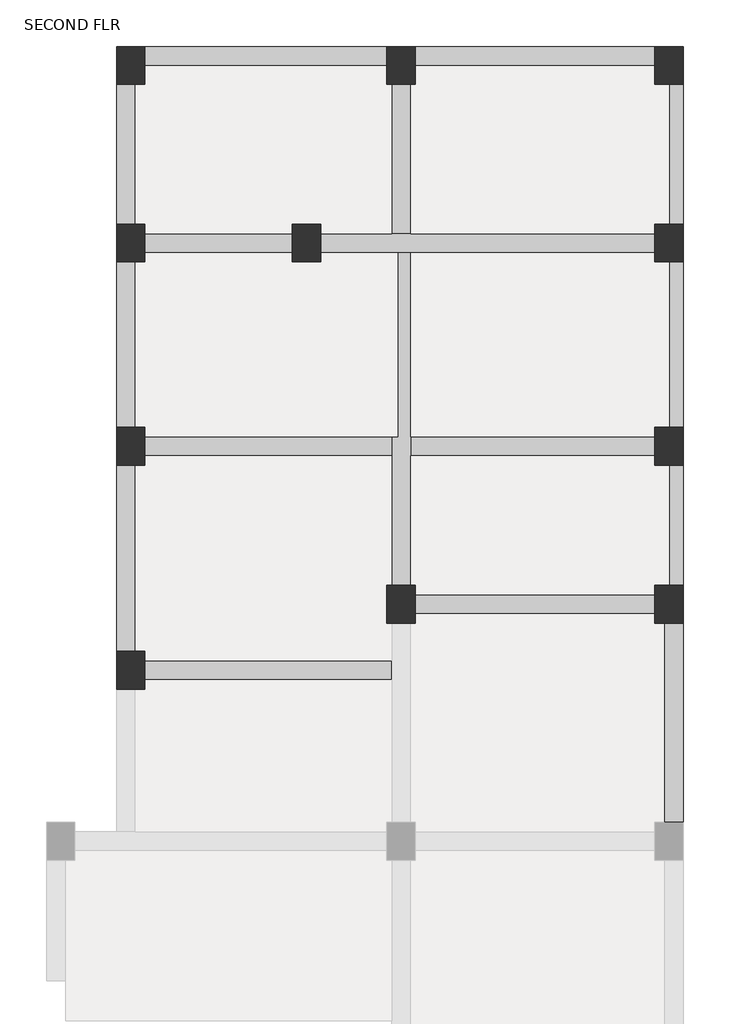
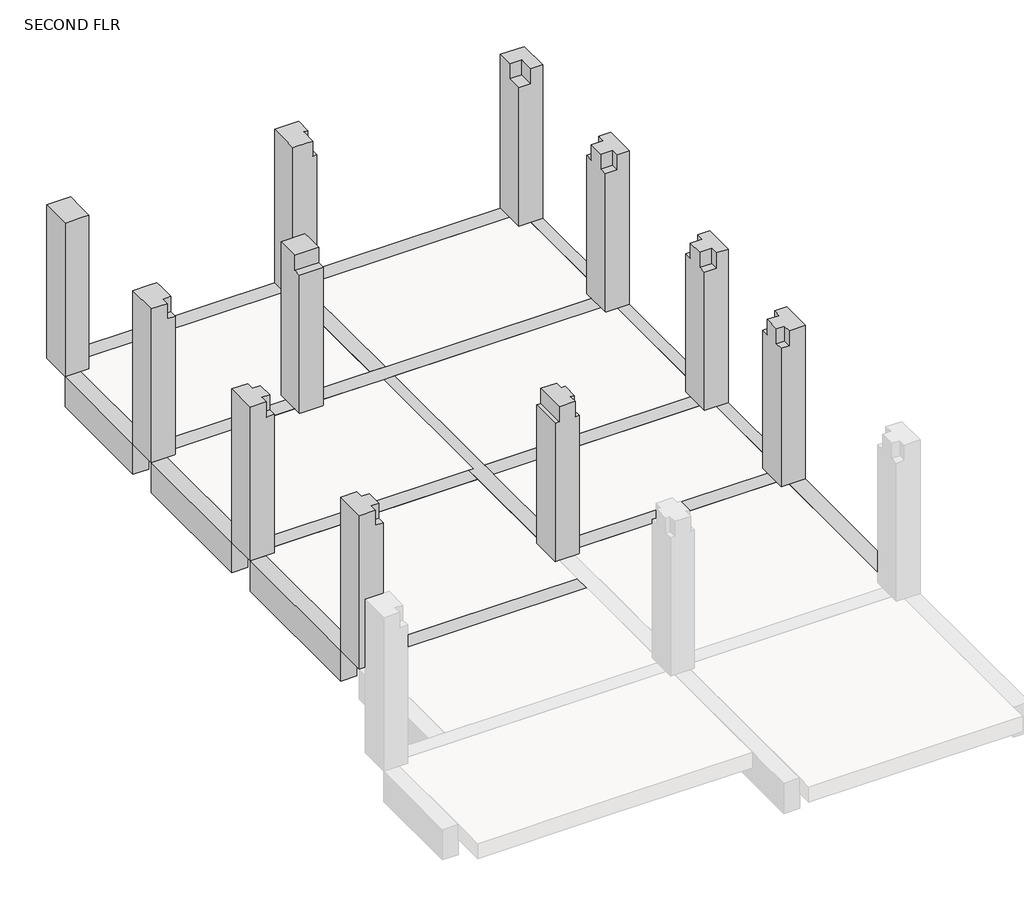
# One storey, part 2 of 2: 17 beams, 11 columns.
"""IFC4 building model written with IfcOpenShell, lengths in millimetres."""

from ifc_helpers import new_model, si_unit, frame, origin, place, context, project, spatial, polyline, outline, extrude, faceted_brep, element, save

model = new_model("IFC4")

# Units and contexts
model_context = context("Model", 3, world=origin())
ifc_project = project(units=[si_unit("LENGTHUNIT", "METRE", prefix="MILLI")], contexts=[model_context])

# Site, building, storey
site = spatial("IfcSite", under=ifc_project)
building = spatial("IfcBuilding", under=site)
storey = spatial("IfcBuildingStorey", under=building, Name="SECOND FLR", Elevation=6048.0)

# Beams
placement = place(None, origin())
element("IfcBeam", 1, ObjectType="M_Concrete-Rectangular Beam : 300 x 600mm", at=placement, inside=storey, context=model_context, shape_type="Brep", body=[
    faceted_brep([(-2096.635935, 10150.0657956, 6048.0), (-2096.635935, 10450.0657956, 6048.0), (-5925.9642664, 10450.0657956, 6048.0), (-5925.9642664, 10150.0657956, 6048.0), (-2096.635935, 10150.0657956, 5448.0), (-2096.635935, 10150.0657956, 5748.0), (-5925.9642664, 10150.0657956, 5748.0), (-5925.9642664, 10150.0657956, 5448.0), (-2096.635935, 10450.0657956, 5448.0), (-5925.9642664, 10450.0657956, 5448.0)], [[[0, 1, 2, 3]], [[4, 5, 0, 3, 6, 7]], [[8, 4, 7, 9]], [[1, 8, 9, 2]], [[2, 9, 7, 6, 3]], [[1, 0, 5, 4, 8]]]),
])
element("IfcBeam", 2, ObjectType="M_Concrete-Rectangular Beam : 300 x 600mm", at=placement, inside=storey, context=model_context, shape_type="SweptSolid", body=[
    extrude(outline(polyline([(2143.5134108, 10450.0657956), (2143.5134108, 10150.0657956), (-1646.635935, 10150.0657956), (-1646.635935, 10450.0657956), (2143.5134108, 10450.0657956)])), frame((0.0, 0.0, 5448.0), z_axis=(0.0, 0.0, 1.0), x_axis=(1.0, 0.0, 0.0)), (0.0, 0.0, 1.0), 600.0),
])
element("IfcBeam", 3, ObjectType="M_Concrete-Rectangular Beam : 300 x 600mm", at=placement, inside=storey, context=model_context, shape_type="Brep", body=[
    faceted_brep([(-6375.9642664, 7641.506653, 6048.0), (-6075.9642664, 7641.506653, 6048.0), (-6075.9642664, 9850.0657956, 6048.0), (-6375.9642664, 9850.0657956, 6048.0), (-6375.9642664, 7641.506653, 5448.0), (-6375.9642664, 9850.0657956, 5448.0), (-6075.9642664, 7641.506653, 5448.0), (-6075.9642664, 9850.0657956, 5448.0), (-6075.9642664, 7641.506653, 5748.0), (-6075.9642664, 9850.0657956, 5748.0)], [[[0, 1, 2, 3]], [[4, 0, 3, 5]], [[6, 4, 5, 7]], [[1, 8, 6, 7, 9, 2]], [[2, 9, 7, 5, 3]], [[1, 0, 4, 6, 8]]]),
])
element("IfcBeam", 4, ObjectType="M_Concrete-Rectangular Beam : 300 x 600mm", at=placement, inside=storey, context=model_context, shape_type="SweptSolid", body=[
    extrude(outline(polyline([(-6075.9642664, 4424.5351605), (-6375.9642664, 4424.5351605), (-6375.9642664, 7041.506653), (-6075.9642664, 7041.506653), (-6075.9642664, 4424.5351605)])), frame((0.0, 0.0, 5448.0), z_axis=(0.0, 0.0, 1.0), x_axis=(1.0, 0.0, 0.0)), (0.0, 0.0, 1.0), 600.0),
])
element("IfcBeam", 5, ObjectType="M_Concrete-Rectangular Beam : 300 x 600mm", at=placement, inside=storey, context=model_context, shape_type="SweptSolid", body=[
    extrude(outline(polyline([(-6075.9642664, 881.5941646), (-6375.9642664, 881.5941646), (-6375.9642664, 3824.5351605), (-6075.9642664, 3824.5351605), (-6075.9642664, 881.5941646)])), frame((0.0, 0.0, 5448.0), z_axis=(0.0, 0.0, 1.0), x_axis=(1.0, 0.0, 0.0)), (0.0, 0.0, 1.0), 600.0),
])
element("IfcBeam", 6, ObjectType="M_Concrete-Rectangular Beam : 300 x 600mm", at=placement, inside=storey, context=model_context, shape_type="SweptSolid", body=[
    extrude(outline(polyline([(2293.5134108, 1328.1057379), (2593.5134108, 1328.1057379), (2593.5134108, -1823.3693625), (2293.5134108, -1823.3693625), (2293.5134108, 1328.1057379)])), frame((0.0, 0.0, 5448.0), z_axis=(0.0, 0.0, 1.0), x_axis=(1.0, 0.0, 0.0)), (0.0, 0.0, 1.0), 600.0),
])
element("IfcBeam", 7, ObjectType="M_Concrete-Rectangular Beam : 300 x 600mm", at=placement, inside=storey, context=model_context, shape_type="SweptSolid", body=[
    extrude(outline(polyline([(5448.0, 2293.5134108), (5448.0, 2593.5134108), (6048.0, 2593.5134108), (6048.0, 2368.5134108), (5748.0, 2368.5134108), (5748.0, 2293.5134108), (5448.0, 2293.5134108)])), frame((0.0, 1928.1057379, 0.0), z_axis=(0.0, 1.0, 0.0), x_axis=(0.0, 0.0, 1.0)), (0.0, 0.0, 1.0), 1896.4294226),
])
element("IfcBeam", 8, ObjectType="M_Concrete-Rectangular Beam : 300 x 600mm", at=placement, inside=storey, context=model_context, shape_type="SweptSolid", body=[
    extrude(outline(polyline([(5448.0, 2293.5134108), (5448.0, 2593.5134108), (6048.0, 2593.5134108), (6048.0, 2368.5134108), (5748.0, 2368.5134108), (5748.0, 2293.5134108), (5448.0, 2293.5134108)])), frame((0.0, 4424.5351605, 0.0), z_axis=(0.0, 1.0, 0.0), x_axis=(0.0, 0.0, 1.0)), (0.0, 0.0, 1.0), 2616.9714925),
])
element("IfcBeam", 9, ObjectType="M_Concrete-Rectangular Beam : 300 x 600mm", at=placement, inside=storey, context=model_context, shape_type="SweptSolid", body=[
    extrude(outline(polyline([(5448.0, 2293.5134108), (5448.0, 2593.5134108), (6048.0, 2593.5134108), (6048.0, 2368.5134108), (5748.0, 2368.5134108), (5748.0, 2293.5134108), (5448.0, 2293.5134108)])), frame((0.0, 7641.506653, 0.0), z_axis=(0.0, 1.0, 0.0), x_axis=(0.0, 0.0, 1.0)), (0.0, 0.0, 1.0), 2208.5591426),
])
element("IfcBeam", 10, ObjectType="M_Concrete-Rectangular Beam : 300 x 600mm", at=placement, inside=storey, context=model_context, shape_type="Brep", body=[
    faceted_brep([(-3596.635935, 7191.506653, 6048.0), (-3596.635935, 7491.506653, 6048.0), (-5925.9642664, 7491.506653, 6048.0), (-5925.9642664, 7191.506653, 6048.0), (-3596.635935, 7191.506653, 5448.0), (-5925.9642664, 7191.506653, 5448.0), (-3596.635935, 7491.506653, 5448.0), (-5925.9642664, 7491.506653, 5448.0), (-3596.635935, 7491.506653, 5748.0), (-5925.9642664, 7491.506653, 5748.0)], [[[0, 1, 2, 3]], [[4, 0, 3, 5]], [[6, 4, 5, 7]], [[1, 8, 6, 7, 9, 2]], [[2, 9, 7, 5, 3]], [[1, 0, 4, 6, 8]]]),
])
element("IfcBeam", 11, ObjectType="M_Concrete-Rectangular Beam : 300 x 600mm", at=placement, inside=storey, context=model_context, shape_type="Brep", body=[
    faceted_brep([(-3146.635935, 7491.506653, 6048.0), (-3146.635935, 7191.506653, 6048.0), (-1928.7254278, 7191.506653, 6048.0), (-1721.635935, 7191.506653, 6048.0), (2143.5134108, 7191.506653, 6048.0), (2143.5134108, 7491.506653, 6048.0), (-1721.635935, 7491.506653, 6048.0), (-2021.635935, 7491.506653, 6048.0), (-3146.635935, 7491.506653, 5448.0), (-3146.635935, 7491.506653, 5748.0), (2143.5134108, 7491.506653, 5448.0), (-1721.635935, 7491.506653, 5448.0), (-2021.635935, 7491.506653, 5448.0), (-3146.635935, 7191.506653, 5448.0), (2143.5134108, 7191.506653, 5448.0), (-1721.635935, 7191.506653, 5448.0), (-2021.635935, 7191.506653, 5448.0)], [[[0, 1, 2, 3, 4, 5, 6, 7]], [[8, 9, 0, 7, 6, 5, 10, 11, 12]], [[13, 8, 12, 11, 10, 14, 15, 16]], [[1, 13, 16, 15, 14, 4, 3, 2]], [[1, 0, 9, 8, 13]], [[4, 14, 10, 5]]]),
])
element("IfcBeam", 12, ObjectType="M_Concrete-Rectangular Beam : 300 x 600mm", at=placement, inside=storey, context=model_context, shape_type="SweptSolid", body=[
    extrude(outline(polyline([(-1646.635935, 1478.1057379), (-1646.635935, 1778.1057379), (2143.5134108, 1778.1057379), (2143.5134108, 1478.1057379), (-1646.635935, 1478.1057379)])), frame((0.0, 0.0, 5448.0), z_axis=(0.0, 0.0, 1.0), x_axis=(1.0, 0.0, 0.0)), (0.0, 0.0, 1.0), 600.0),
])
element("IfcBeam", 13, ObjectType="M_Concrete-Rectangular Beam : 300 x 600mm", at=placement, inside=storey, context=model_context, shape_type="Brep", body=[
    faceted_brep([(-1721.635935, 9850.0657956, 6048.0), (-2021.635935, 9850.0657956, 6048.0), (-2021.635935, 7491.506653, 6048.0), (-1721.635935, 7491.506653, 6048.0), (-2021.635935, 9850.0657956, 5748.0), (-2021.635935, 9850.0657956, 5448.0), (-2021.635935, 7491.506653, 5448.0), (-2021.635935, 7491.506653, 5748.0), (-1721.635935, 9850.0657956, 5448.0), (-1721.635935, 7491.506653, 5448.0), (-1721.635935, 7491.506653, 5748.0)], [[[0, 1, 2, 3]], [[1, 4, 5, 6, 7, 2]], [[5, 8, 9, 6]], [[8, 0, 3, 10, 9]], [[0, 8, 5, 4, 1]], [[3, 2, 7, 6, 9, 10]]]),
])
element("IfcBeam", 14, ObjectType="M_Concrete-Rectangular Beam : 300 x 600mm", at=placement, inside=storey, context=model_context, shape_type="Brep", body=[
    faceted_brep([(-2021.635935, 1928.1057379, 6048.0), (-1721.635935, 1928.1057379, 6048.0), (-1721.635935, 3974.5351605, 6048.0), (-1721.635935, 4274.5351605, 6048.0), (-1721.635935, 7191.506653, 6048.0), (-1928.7254278, 7191.506653, 6048.0), (-1928.7254278, 4274.5351605, 6048.0), (-2021.635935, 4274.5351605, 6048.0), (-2021.635935, 3974.5351605, 6048.0), (-1721.635935, 1928.1057379, 5448.0), (-1721.635935, 3974.5351605, 5448.0), (-1721.635935, 4274.5351605, 5448.0), (-1721.635935, 7191.506653, 5448.0), (-1721.635935, 7191.506653, 5748.0), (-2021.635935, 1928.1057379, 5448.0), (-2021.635935, 3974.5351605, 5448.0), (-2021.635935, 4274.5351605, 5448.0), (-2021.635935, 7191.506653, 5448.0), (-2021.635935, 4274.5351605, 5748.0), (-2021.635935, 7191.506653, 5748.0), (-1928.7254278, 7191.506653, 5748.0), (-1928.7254278, 4274.5351605, 5748.0)], [[[0, 1, 2, 3, 4, 5, 6, 7, 8]], [[1, 9, 10, 11, 12, 13, 4, 3, 2]], [[9, 14, 15, 16, 17, 12, 11, 10]], [[14, 0, 8, 7, 18, 19, 17, 16, 15]], [[0, 14, 9, 1]], [[4, 13, 12, 17, 19, 20, 5]], [[21, 20, 19, 18]], [[20, 21, 6, 5]], [[6, 21, 18, 7]]]),
])
element("IfcBeam", 15, ObjectType="M_Concrete-Rectangular Beam : 300 x 600mm", at=placement, inside=storey, context=model_context, shape_type="Brep", body=[
    faceted_brep([(-5925.9642664, 731.5941646, 6048.0), (-5925.9642664, 431.5941646, 6048.0), (-2021.635935, 431.5941646, 6048.0), (-2021.635935, 731.5941646, 6048.0), (-5925.9642664, 431.5941646, 5448.0), (-2021.635935, 431.5941646, 5448.0), (-2021.635935, 431.5941646, 5748.0), (-5925.9642664, 731.5941646, 5448.0), (-2021.635935, 731.5941646, 5448.0), (-2021.635935, 731.5941646, 5748.0)], [[[0, 1, 2, 3]], [[1, 4, 5, 6, 2]], [[4, 7, 8, 5]], [[7, 0, 3, 9, 8]], [[0, 7, 4, 1]], [[3, 2, 6, 5, 8, 9]]]),
])
element("IfcBeam", 16, ObjectType="M_Concrete-Rectangular Beam : 300 x 600mm", at=placement, inside=storey, context=model_context, shape_type="Brep", body=[
    faceted_brep([(-5925.9642664, 4274.5351605, 6048.0), (-5925.9642664, 3974.5351605, 6048.0), (-2021.635935, 3974.5351605, 6048.0), (-2021.635935, 4274.5351605, 6048.0), (-5925.9642664, 3974.5351605, 5448.0), (-2021.635935, 3974.5351605, 5448.0), (-2021.635935, 3974.5351605, 5748.0), (-5925.9642664, 4274.5351605, 5448.0), (-2021.635935, 4274.5351605, 5448.0), (-2021.635935, 4274.5351605, 5748.0)], [[[0, 1, 2, 3]], [[1, 4, 5, 6, 2]], [[4, 7, 8, 5]], [[7, 0, 3, 9, 8]], [[0, 7, 4, 1]], [[3, 2, 6, 5, 8, 9]]]),
])
element("IfcBeam", 17, ObjectType="M_Concrete-Rectangular Beam : 300 x 600mm", at=placement, inside=storey, context=model_context, shape_type="Brep", body=[
    faceted_brep([(2143.5134108, 3974.5351605, 6048.0), (2143.5134108, 4274.5351605, 6048.0), (-1721.635935, 4274.5351605, 6048.0), (-1721.635935, 3974.5351605, 6048.0), (2143.5134108, 4274.5351605, 5448.0), (-1721.635935, 4274.5351605, 5448.0), (-1721.635935, 4274.5351605, 5748.0), (2143.5134108, 3974.5351605, 5448.0), (-1721.635935, 3974.5351605, 5448.0), (-1721.635935, 3974.5351605, 5748.0)], [[[0, 1, 2, 3]], [[1, 4, 5, 6, 2]], [[4, 7, 8, 5]], [[7, 0, 3, 9, 8]], [[0, 7, 4, 1]], [[3, 2, 6, 5, 8, 9]]]),
])

# Columns
element("IfcColumn", 18, ObjectType="M_Concrete-Rectangular-Column : 450 x 600mm", at=placement, inside=storey, context=model_context, shape_type="Brep", body=[
    faceted_brep([(-5925.9642664, 10450.0657956, 6048.0), (-5925.9642664, 9850.0657956, 6048.0), (-6375.9642664, 9850.0657956, 6048.0), (-6375.9642664, 10450.0657956, 6048.0), (-5925.9642664, 10450.0657956, 9096.0), (-5925.9642664, 10150.0657956, 9096.0), (-5925.9642664, 9850.0657956, 9096.0), (-5925.9642664, 9850.0657956, 8796.0), (-6075.9642664, 9850.0657956, 9096.0), (-6375.9642664, 9850.0657956, 9096.0), (-6375.9642664, 10450.0657956, 9096.0)], [[[0, 1, 2, 3]], [[1, 0, 4, 5, 6, 7]], [[2, 1, 7, 6, 8, 9]], [[3, 2, 9, 10]], [[0, 3, 10, 4]], [[10, 9, 8, 6, 5, 4]]]),
])
element("IfcColumn", 19, ObjectType="M_Concrete-Rectangular-Column : 450 x 600mm", at=placement, inside=storey, context=model_context, shape_type="Brep", body=[
    faceted_brep([(-5925.9642664, 7641.506653, 6048.0), (-5925.9642664, 7041.506653, 6048.0), (-6375.9642664, 7041.506653, 6048.0), (-6375.9642664, 7641.506653, 6048.0), (-5925.9642664, 7641.506653, 8796.0), (-5925.9642664, 7641.506653, 9096.0), (-5925.9642664, 7491.506653, 9096.0), (-5925.9642664, 7191.506653, 9096.0), (-5925.9642664, 7191.506653, 8796.0), (-5925.9642664, 7041.506653, 8796.0), (-6075.9642664, 7041.506653, 8796.0), (-6075.9642664, 7041.506653, 9096.0), (-6375.9642664, 7041.506653, 9096.0), (-6375.9642664, 7641.506653, 9096.0), (-6075.9642664, 7641.506653, 9096.0), (-6075.9642664, 7191.506653, 9096.0), (-6075.9642664, 7191.506653, 8796.0)], [[[0, 1, 2, 3]], [[1, 0, 4, 5, 6, 7, 8, 9]], [[2, 1, 9, 10, 11, 12]], [[3, 2, 12, 13]], [[0, 3, 13, 14, 5, 4]], [[13, 12, 11, 15, 7, 6, 5, 14]], [[16, 10, 9, 8]], [[15, 16, 8, 7]], [[16, 15, 11, 10]]]),
])
element("IfcColumn", 20, ObjectType="M_Concrete-Rectangular-Column : 450 x 600mm", at=placement, inside=storey, context=model_context, shape_type="Brep", body=[
    faceted_brep([(-5925.9642664, 4424.5351605, 6048.0), (-5925.9642664, 3824.5351605, 6048.0), (-6375.9642664, 3824.5351605, 6048.0), (-6375.9642664, 4424.5351605, 6048.0), (-5925.9642664, 4424.5351605, 8796.0), (-5925.9642664, 4274.5351605, 8796.0), (-5925.9642664, 4274.5351605, 9096.0), (-5925.9642664, 3974.5351605, 9096.0), (-5925.9642664, 3974.5351605, 8796.0), (-5925.9642664, 3824.5351605, 8796.0), (-6075.9642664, 3824.5351605, 8796.0), (-6075.9642664, 3824.5351605, 9096.0), (-6375.9642664, 3824.5351605, 9096.0), (-6375.9642664, 4424.5351605, 9096.0), (-6075.9642664, 4424.5351605, 9096.0), (-6075.9642664, 4424.5351605, 8796.0), (-6075.9642664, 3974.5351605, 9096.0), (-6075.9642664, 4274.5351605, 9096.0), (-6075.9642664, 4274.5351605, 8796.0), (-6075.9642664, 3974.5351605, 8796.0)], [[[0, 1, 2, 3]], [[1, 0, 4, 5, 6, 7, 8, 9]], [[2, 1, 9, 10, 11, 12]], [[3, 2, 12, 13]], [[0, 3, 13, 14, 15, 4]], [[13, 12, 11, 16, 7, 6, 17, 14]], [[15, 18, 5, 4]], [[18, 17, 6, 5]], [[17, 18, 15, 14]], [[19, 10, 9, 8]], [[16, 19, 8, 7]], [[19, 16, 11, 10]]]),
])
element("IfcColumn", 21, ObjectType="M_Concrete-Rectangular-Column : 450 x 600mm", at=placement, inside=storey, context=model_context, shape_type="Brep", body=[
    faceted_brep([(-5925.9642664, 881.5941646, 6048.0), (-5925.9642664, 281.5941646, 6048.0), (-6375.9642664, 281.5941646, 6048.0), (-6375.9642664, 881.5941646, 6048.0), (-5925.9642664, 881.5941646, 8796.0), (-5925.9642664, 731.5941646, 8796.0), (-5925.9642664, 731.5941646, 9096.0), (-5925.9642664, 431.5941646, 9096.0), (-5925.9642664, 431.5941646, 8796.0), (-5925.9642664, 281.5941646, 8796.0), (-6075.9642664, 281.5941646, 8796.0), (-6075.9642664, 281.5941646, 9096.0), (-6375.9642664, 281.5941646, 9096.0), (-6375.9642664, 881.5941646, 9096.0), (-6075.9642664, 881.5941646, 9096.0), (-6075.9642664, 881.5941646, 8796.0), (-6075.9642664, 431.5941646, 9096.0), (-6075.9642664, 731.5941646, 9096.0), (-6075.9642664, 731.5941646, 8796.0), (-6075.9642664, 431.5941646, 8796.0)], [[[0, 1, 2, 3]], [[1, 0, 4, 5, 6, 7, 8, 9]], [[2, 1, 9, 10, 11, 12]], [[3, 2, 12, 13]], [[0, 3, 13, 14, 15, 4]], [[13, 12, 11, 16, 7, 6, 17, 14]], [[15, 18, 5, 4]], [[18, 17, 6, 5]], [[17, 18, 15, 14]], [[19, 10, 9, 8]], [[19, 16, 11, 10]], [[16, 19, 8, 7]]]),
])
element("IfcColumn", 22, ObjectType="M_Concrete-Rectangular-Column : 450 x 600mm", at=placement, inside=storey, context=model_context, shape_type="Brep", body=[
    faceted_brep([(-3146.635935, 7641.506653, 6048.0), (-3146.635935, 7041.506653, 6048.0), (-3596.635935, 7041.506653, 6048.0), (-3596.635935, 7641.506653, 6048.0), (-3146.635935, 7641.506653, 8796.0), (-3146.635935, 7641.506653, 9096.0), (-3146.635935, 7491.506653, 9096.0), (-3146.635935, 7191.506653, 9096.0), (-3146.635935, 7191.506653, 8796.0), (-3146.635935, 7041.506653, 8796.0), (-3596.635935, 7041.506653, 8796.0), (-3596.635935, 7191.506653, 8796.0), (-3596.635935, 7191.506653, 9096.0), (-3596.635935, 7491.506653, 9096.0), (-3596.635935, 7641.506653, 9096.0), (-3596.635935, 7641.506653, 8796.0)], [[[0, 1, 2, 3]], [[1, 0, 4, 5, 6, 7, 8, 9]], [[2, 1, 9, 10]], [[3, 2, 10, 11, 12, 13, 14, 15]], [[0, 3, 15, 14, 5, 4]], [[5, 14, 13, 12, 7, 6]], [[8, 11, 10, 9]], [[11, 8, 7, 12]]]),
])
element("IfcColumn", 23, ObjectType="M_Concrete-Rectangular-Column : 450 x 600mm", at=placement, inside=storey, context=model_context, shape_type="Brep", body=[
    faceted_brep([(-1646.635935, 10450.0657956, 6048.0), (-1646.635935, 9850.0657956, 6048.0), (-2096.635935, 9850.0657956, 6048.0), (-2096.635935, 10450.0657956, 6048.0), (-1646.635935, 10450.0657956, 9096.0), (-1646.635935, 10150.0657956, 9096.0), (-1646.635935, 10150.0657956, 8796.0), (-1646.635935, 9850.0657956, 8796.0), (-1721.635935, 9850.0657956, 8796.0), (-1721.635935, 9850.0657956, 9096.0), (-2021.635935, 9850.0657956, 9096.0), (-2096.635935, 9850.0657956, 9096.0), (-2096.635935, 9850.0657956, 8796.0), (-2096.635935, 10150.0657956, 9096.0), (-2096.635935, 10450.0657956, 9096.0), (-1721.635935, 10150.0657956, 9096.0), (-1721.635935, 10150.0657956, 8796.0)], [[[0, 1, 2, 3]], [[1, 0, 4, 5, 6, 7]], [[2, 1, 7, 8, 9, 10, 11, 12]], [[3, 2, 12, 11, 13, 14]], [[0, 3, 14, 4]], [[4, 14, 13, 11, 10, 9, 15, 5]], [[16, 8, 7, 6]], [[15, 16, 6, 5]], [[16, 15, 9, 8]]]),
])
element("IfcColumn", 24, ObjectType="M_Concrete-Rectangular-Column : 450 x 600mm", at=placement, inside=storey, context=model_context, shape_type="Brep", body=[
    faceted_brep([(-1646.635935, 1928.1057379, 6048.0), (-1646.635935, 1328.1057379, 6048.0), (-2096.635935, 1328.1057379, 6048.0), (-2096.635935, 1928.1057379, 6048.0), (-1646.635935, 1928.1057379, 8796.0), (-1646.635935, 1778.1057379, 8796.0), (-1646.635935, 1778.1057379, 9096.0), (-1646.635935, 1478.1057379, 9096.0), (-1646.635935, 1478.1057379, 8796.0), (-1646.635935, 1328.1057379, 8796.0), (-1721.635935, 1328.1057379, 8796.0), (-1721.635935, 1328.1057379, 9096.0), (-2021.635935, 1328.1057379, 9096.0), (-2021.635935, 1328.1057379, 8796.0), (-2096.635935, 1328.1057379, 8796.0), (-2096.635935, 1928.1057379, 8796.0), (-2021.635935, 1928.1057379, 8796.0), (-2021.635935, 1928.1057379, 9096.0), (-1721.635935, 1928.1057379, 9096.0), (-1721.635935, 1928.1057379, 8796.0), (-1721.635935, 1778.1057379, 9096.0), (-1721.635935, 1478.1057379, 9096.0), (-1721.635935, 1778.1057379, 8796.0), (-1721.635935, 1478.1057379, 8796.0)], [[[0, 1, 2, 3]], [[1, 0, 4, 5, 6, 7, 8, 9]], [[2, 1, 9, 10, 11, 12, 13, 14]], [[3, 2, 14, 15]], [[0, 3, 15, 16, 17, 18, 19, 4]], [[6, 20, 18, 17, 12, 11, 21, 7]], [[19, 22, 5, 4]], [[22, 20, 6, 5]], [[20, 22, 19, 18]], [[23, 10, 9, 8]], [[21, 23, 8, 7]], [[23, 21, 11, 10]], [[13, 16, 15, 14]], [[16, 13, 12, 17]]]),
])
element("IfcColumn", 25, ObjectType="M_Concrete-Rectangular-Column : 450 x 600mm", at=placement, inside=storey, context=model_context, shape_type="Brep", body=[
    faceted_brep([(2593.5134108, 10450.0657956, 6048.0), (2593.5134108, 9850.0657956, 6048.0), (2143.5134108, 9850.0657956, 6048.0), (2143.5134108, 10450.0657956, 6048.0), (2593.5134108, 10450.0657956, 9096.0), (2593.5134108, 9850.0657956, 9096.0), (2368.5134108, 9850.0657956, 9096.0), (2368.5134108, 9850.0657956, 8796.0), (2143.5134108, 9850.0657956, 8796.0), (2143.5134108, 10150.0657956, 8796.0), (2143.5134108, 10150.0657956, 9096.0), (2143.5134108, 10450.0657956, 9096.0), (2368.5134108, 10150.0657956, 9096.0), (2368.5134108, 10150.0657956, 8796.0)], [[[0, 1, 2, 3]], [[1, 0, 4, 5]], [[2, 1, 5, 6, 7, 8]], [[3, 2, 8, 9, 10, 11]], [[0, 3, 11, 4]], [[5, 4, 11, 10, 12, 6]], [[7, 13, 9, 8]], [[13, 12, 10, 9]], [[12, 13, 7, 6]]]),
])
element("IfcColumn", 26, ObjectType="M_Concrete-Rectangular-Column : 450 x 600mm", at=placement, inside=storey, context=model_context, shape_type="Brep", body=[
    faceted_brep([(2593.5134108, 7641.506653, 6048.0), (2593.5134108, 7041.506653, 6048.0), (2143.5134108, 7041.506653, 6048.0), (2143.5134108, 7641.506653, 6048.0), (2593.5134108, 7641.506653, 9096.0), (2593.5134108, 7041.506653, 9096.0), (2368.5134108, 7041.506653, 9096.0), (2368.5134108, 7041.506653, 8796.0), (2143.5134108, 7041.506653, 8796.0), (2143.5134108, 7191.506653, 8796.0), (2143.5134108, 7191.506653, 9096.0), (2143.5134108, 7491.506653, 9096.0), (2143.5134108, 7491.506653, 8796.0), (2143.5134108, 7641.506653, 8796.0), (2368.5134108, 7641.506653, 8796.0), (2368.5134108, 7641.506653, 9096.0), (2368.5134108, 7491.506653, 9096.0), (2368.5134108, 7191.506653, 9096.0), (2368.5134108, 7491.506653, 8796.0), (2368.5134108, 7191.506653, 8796.0)], [[[0, 1, 2, 3]], [[1, 0, 4, 5]], [[2, 1, 5, 6, 7, 8]], [[3, 2, 8, 9, 10, 11, 12, 13]], [[0, 3, 13, 14, 15, 4]], [[5, 4, 15, 16, 11, 10, 17, 6]], [[12, 18, 14, 13]], [[18, 16, 15, 14]], [[16, 18, 12, 11]], [[7, 19, 9, 8]], [[19, 17, 10, 9]], [[17, 19, 7, 6]]]),
])
element("IfcColumn", 27, ObjectType="M_Concrete-Rectangular-Column : 450 x 600mm", at=placement, inside=storey, context=model_context, shape_type="Brep", body=[
    faceted_brep([(2593.5134108, 4424.5351605, 6048.0), (2593.5134108, 3824.5351605, 6048.0), (2143.5134108, 3824.5351605, 6048.0), (2143.5134108, 4424.5351605, 6048.0), (2593.5134108, 4424.5351605, 9096.0), (2593.5134108, 3824.5351605, 9096.0), (2368.5134108, 3824.5351605, 9096.0), (2368.5134108, 3824.5351605, 8796.0), (2143.5134108, 3824.5351605, 8796.0), (2143.5134108, 3974.5351605, 8796.0), (2143.5134108, 3974.5351605, 9096.0), (2143.5134108, 4274.5351605, 9096.0), (2143.5134108, 4274.5351605, 8796.0), (2143.5134108, 4424.5351605, 8796.0), (2368.5134108, 4424.5351605, 8796.0), (2368.5134108, 4424.5351605, 9096.0), (2368.5134108, 4274.5351605, 9096.0), (2368.5134108, 3974.5351605, 9096.0), (2368.5134108, 4274.5351605, 8796.0), (2368.5134108, 3974.5351605, 8796.0)], [[[0, 1, 2, 3]], [[1, 0, 4, 5]], [[2, 1, 5, 6, 7, 8]], [[3, 2, 8, 9, 10, 11, 12, 13]], [[0, 3, 13, 14, 15, 4]], [[5, 4, 15, 16, 11, 10, 17, 6]], [[12, 18, 14, 13]], [[18, 16, 15, 14]], [[16, 18, 12, 11]], [[7, 19, 9, 8]], [[17, 19, 7, 6]], [[19, 17, 10, 9]]]),
])
element("IfcColumn", 28, ObjectType="M_Concrete-Rectangular-Column : 450 x 600mm", at=placement, inside=storey, context=model_context, shape_type="Brep", body=[
    faceted_brep([(2593.5134108, 1928.1057379, 6048.0), (2593.5134108, 1328.1057379, 6048.0), (2143.5134108, 1328.1057379, 6048.0), (2143.5134108, 1928.1057379, 6048.0), (2593.5134108, 1928.1057379, 9096.0), (2593.5134108, 1328.1057379, 9096.0), (2293.5134108, 1328.1057379, 9096.0), (2293.5134108, 1328.1057379, 8796.0), (2143.5134108, 1328.1057379, 8796.0), (2143.5134108, 1478.1057379, 8796.0), (2143.5134108, 1478.1057379, 9096.0), (2143.5134108, 1778.1057379, 9096.0), (2143.5134108, 1778.1057379, 8796.0), (2143.5134108, 1928.1057379, 8796.0), (2368.5134108, 1928.1057379, 8796.0), (2368.5134108, 1928.1057379, 9096.0), (2368.5134108, 1778.1057379, 9096.0), (2293.5134108, 1478.1057379, 9096.0), (2368.5134108, 1778.1057379, 8796.0), (2293.5134108, 1478.1057379, 8796.0)], [[[0, 1, 2, 3]], [[1, 0, 4, 5]], [[2, 1, 5, 6, 7, 8]], [[3, 2, 8, 9, 10, 11, 12, 13]], [[0, 3, 13, 14, 15, 4]], [[5, 4, 15, 16, 11, 10, 17, 6]], [[12, 18, 14, 13]], [[18, 16, 15, 14]], [[16, 18, 12, 11]], [[7, 19, 9, 8]], [[19, 17, 10, 9]], [[17, 19, 7, 6]]]),
])

save(model, "model.ifc")

# Revit data of these elements
# Type "M_Concrete-Rectangular Beam : 300 x 600mm"
#   Length [instance default] = 1524 mm
#   b = 300 mm
#   h = 600 mm
#   Structural Material [instance default] = Concrete, Cast-in-Place gray
#   Assembly Code = ""
# Type "M_Concrete-Rectangular-Column : 450 x 600mm"
#   b = 450 mm
#   h = 600 mm
#   Structural Material [instance default] = Concrete, Cast-in-Place gray
# Elements 1, 2, 3, 4, 5, 6, 7, 8, 9, 10, 11, 12, 13, 14, 15, 16, 17 (IfcBeam, "M_Concrete-Rectangular Beam : 300 x 600mm")
#   Structural Material = Concrete, Cast-in-Place gray
#   Phase Created = New Construction
#   Materials on its faces: "Concrete, Cast-in-Place gray"
# Elements 18, 19, 20, 21, 22, 23, 24, 25, 26, 27, 28 (IfcColumn, "M_Concrete-Rectangular-Column : 450 x 600mm")
#   Structural Material = Concrete, Cast-in-Place gray
#   Phase Created = New Construction
#   Materials on its faces: "Concrete, Cast-in-Place gray"
# Materials
#   "Concrete, Cast-in-Place gray": class "Concrete", colour RGB 192 192 192, transparency 0, Description = "Cast-in-place concrete", Cost = 0
